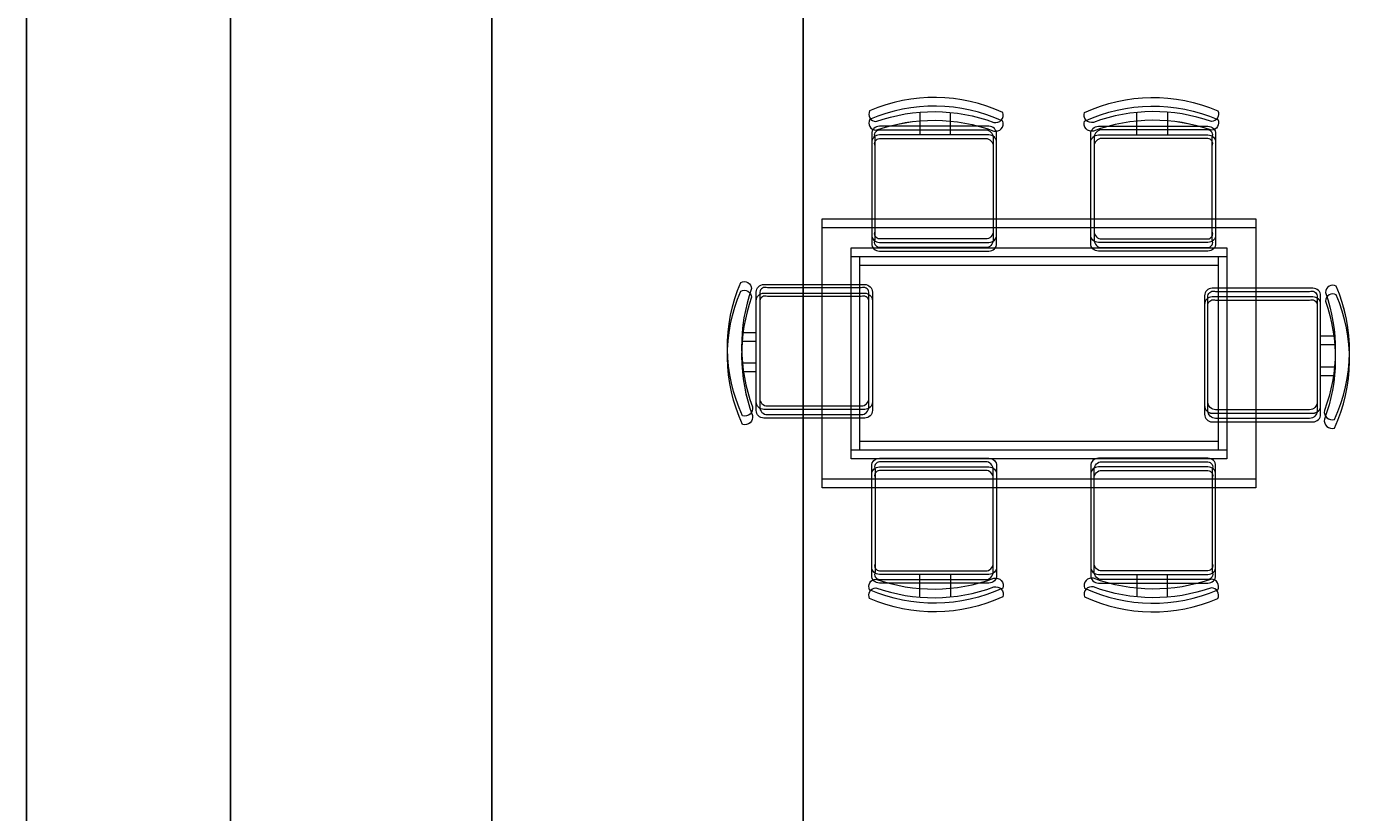
# Model space of a CAD drawing. Units: inches. Extents: x 1601 to 2297, y 1496 to 2631.
# Tile 25 of 57: x 2040 to 2141, y 1887 to 1946. Entities that reach past the tile are written whole.
import ezdxf

# ---------------------------------------------------------------- set-up
doc = ezdxf.new("R2010")
doc.units = ezdxf.units.IN
doc.layers.add('A-ANNO-DIMS', color=2, linetype='Continuous', lineweight=18)
doc.layers.add('A-FURN', color=8, linetype='Continuous', lineweight=18)
doc.styles.get("Standard").update_dxf_attribs({"font": 'arial.ttf'})
doc.dimstyles.get("Standard").update_dxf_attribs({"dimtxt": 0.18, "dimasz": 0.18, "dimexe": 0.18, "dimexo": 0.0625, "dimgap": 0.09, "dimtad": 0, "dimtih": 1, "dimtoh": 1, "dimdec": 4, "dimzin": 0, "dimdsep": 46, "dimtxsty": 'Standard', "dimcen": 0.09, "dimadec": 0, "dimazin": 0, "dimtfac": 1, "dimtdec": 4, "dimtofl": 0, "dimtmove": 0, "dimatfit": 3, "dimfxl": 1, "dimtolj": 1, "dimtzin": 0, "dimarcsym": 0})

# ---------------------------------------------------------------- blocks, each defined once
blk = doc.blocks.new('DINING-TABLE')
for points in [[(0, 20.42), (32.93, 20.42), (32.93, 0.66), (0, 0.66)], [(0, 20.42), (32.93, 20.42), (32.93, 0.66), (0, 0.66)], [(0, 20.42), (32.93, 20.42), (32.93, 0.66), (0, 0.66)], [(0, 20.42), (32.93, 20.42), (32.93, 0.66), (0, 0.66)], [(0, 19.76), (32.93, 19.76), (32.93, 0), (0, 0)], [(0, 19.76), (32.93, 19.76), (32.93, 0), (0, 0)], [(0, 19.76), (32.93, 19.76), (32.93, 0), (0, 0)], [(0, 19.76), (32.93, 19.76), (32.93, 0), (0, 0)], [(2.2, 18.22), (30.73, 18.22), (30.73, 2.85), (2.2, 2.85)], [(2.2, 18.22), (30.73, 18.22), (30.73, 2.85), (2.2, 2.85)], [(2.2, 18.22), (30.73, 18.22), (30.73, 2.85), (2.2, 2.85)], [(2.2, 18.22), (30.73, 18.22), (30.73, 2.85), (2.2, 2.85)], [(2.2, 17.56), (30.73, 17.56), (30.73, 2.2), (2.2, 2.2)], [(2.2, 17.56), (30.73, 17.56), (30.73, 2.2), (2.2, 2.2)], [(2.2, 17.56), (30.73, 17.56), (30.73, 2.2), (2.2, 2.2)], [(2.2, 17.56), (30.73, 17.56), (30.73, 2.2), (2.2, 2.2)], [(2.85, 17.56), (30.08, 17.56), (30.08, 3.51), (2.85, 3.51)], [(2.85, 17.56), (30.08, 17.56), (30.08, 3.51), (2.85, 3.51)], [(2.85, 17.56), (30.08, 17.56), (30.08, 3.51), (2.85, 3.51)], [(2.85, 17.56), (30.08, 17.56), (30.08, 3.51), (2.85, 3.51)], [(2.85, 16.9), (30.08, 16.9), (30.08, 2.85), (2.85, 2.85)], [(2.85, 16.9), (30.08, 16.9), (30.08, 2.85), (2.85, 2.85)], [(2.85, 16.9), (30.08, 16.9), (30.08, 2.85), (2.85, 2.85)], [(2.85, 16.9), (30.08, 16.9), (30.08, 2.85), (2.85, 2.85)]]:
    blk.add_lwpolyline(points, close=True)
blk = doc.blocks.new('*D39')
at = {"layer": 'A-ANNO-DIMS', "color": 0, "lineweight": -2, "transparency": 16777216}
for p, q in [((2055.55, 1981.76), (2055.55, 1513.75)), ((2099.05, 1981.76), (2099.05, 1513.75)), ((2055.73, 1513.93), (2076.97, 1513.93)), ((2098.87, 1513.93), (2077.63, 1513.93))]:
    blk.add_line(p, q, dxfattribs=at)
at = {"layer": 'A-ANNO-DIMS', "color": 0, "transparency": 16777216}
for points in [[(2055.73, 1513.96), (2055.73, 1513.9), (2055.55, 1513.93)], [(2098.87, 1513.96), (2098.87, 1513.9), (2099.05, 1513.93)]]:
    blk.add_solid(points, dxfattribs=at)
at = {"layer": 'Defpoints', "color": 0, "transparency": 16777216}
for p in [(2055.55, 1981.83), (2099.05, 1981.83), (2099.05, 1513.93)]:
    blk.add_point(p, dxfattribs=at)
at = {"layer": 'A-ANNO-DIMS', "color": 0, "transparency": 16777216, "insert": (2077.3, 1513.93), "char_height": 0.18, "attachment_point": 5}
blk.add_mtext('\\A1;43.5', dxfattribs=at)
blk = doc.blocks.new('*D41')
at = {"layer": 'A-ANNO-DIMS', "color": 0, "lineweight": -2, "transparency": 16777216}
for p, q in [((2075.4, 2070.14), (2075.4, 1513.75)), ((2040.04, 2066.51), (2040.04, 1513.75)), ((2040.22, 1513.93), (2057.32, 1513.93)), ((2075.22, 1513.93), (2058.11, 1513.93))]:
    blk.add_line(p, q, dxfattribs=at)
at = {"layer": 'A-ANNO-DIMS', "color": 0, "transparency": 16777216}
for points in [[(2040.22, 1513.96), (2040.22, 1513.9), (2040.04, 1513.93)], [(2075.22, 1513.96), (2075.22, 1513.9), (2075.4, 1513.93)]]:
    blk.add_solid(points, dxfattribs=at)
at = {"layer": 'Defpoints', "color": 0, "transparency": 16777216}
for p in [(2075.4, 2070.2), (2040.04, 2066.58), (2075.4, 1513.93)]:
    blk.add_point(p, dxfattribs=at)
at = {"layer": 'A-ANNO-DIMS', "color": 0, "transparency": 16777216, "insert": (2057.72, 1513.93), "char_height": 0.18, "attachment_point": 5}
blk.add_mtext('\\A1;35.36', dxfattribs=at)

msp = doc.modelspace()

# ---------------------------------------------------------------- linework, layer by layer
at = {"layer": 'A-FURN'}
for points in [[(2104.571, 1939.1051, -0.17580919), (2113.5401, 1939.0371, 0.57839206), (2114.2196, 1939.7843, 0.21452438), (2104.0954, 1939.9201, 0.55201397), (2104.571, 1939.1051, -0.06507904)], [(2104.571, 1939.1051, -0.17580919), (2113.5401, 1939.0371, 0.57839206), (2114.2196, 1939.7843, 0.21452438), (2104.0954, 1939.9201, 0.55201397), (2104.571, 1939.1051, -0.06507904)], [(2104.5711, 1939.1047, -0.17580919), (2113.5401, 1939.0368, 0.57839206), (2114.2196, 1939.7839, 0.21452438), (2104.0954, 1939.9198, 0.55201397), (2104.5711, 1939.1047, -0.06507904)], [(2104.5711, 1939.1047, -0.17580919), (2113.5401, 1939.0368, 0.57839206), (2114.2196, 1939.7839, 0.21452438), (2104.0954, 1939.9198, 0.55201397), (2104.5711, 1939.1047, -0.06507904)], [(2121.0909, 1939.0371, -0.57839206), (2120.4115, 1939.7843, -0.21452438), (2130.5357, 1939.9201, -0.55201397), (2130.06, 1939.1051, 0.1758092), (2121.0909, 1939.0371)], [(2121.0909, 1939.0371, -0.57839206), (2120.4115, 1939.7843, -0.21452438), (2130.5357, 1939.9201, -0.55201397), (2130.06, 1939.1051, 0.1758092), (2121.0909, 1939.0371)], [(2121.091, 1939.0368, -0.57839206), (2120.4115, 1939.7839, -0.21452438), (2130.5357, 1939.9198, -0.55201397), (2130.06, 1939.1047, 0.1758092), (2121.091, 1939.0368)], [(2121.091, 1939.0368, -0.57839206), (2120.4115, 1939.7839, -0.21452438), (2130.5357, 1939.9198, -0.55201397), (2130.06, 1939.1047, 0.1758092), (2121.091, 1939.0368)], [(2104.571, 1938.4465, -0.17580919), (2113.5401, 1938.3785, 0.57839206), (2114.2196, 1939.1257, 0.21452438), (2104.0954, 1939.2615, 0.55201397), (2104.571, 1938.4465, -0.06507904)], [(2104.571, 1938.4465, -0.17580919), (2113.5401, 1938.3785, 0.57839206), (2114.2196, 1939.1257, 0.21452438), (2104.0954, 1939.2615, 0.55201397), (2104.571, 1938.4465, -0.06507904)], [(2104.5711, 1938.4461, -0.17580919), (2113.5401, 1938.3782, 0.57839206), (2114.2196, 1939.1253, 0.21452438), (2104.0954, 1939.2612, 0.55201397), (2104.5711, 1938.4461, -0.06507904)], [(2104.5711, 1938.4461, -0.17580919), (2113.5401, 1938.3782, 0.57839206), (2114.2196, 1939.1253, 0.21452438), (2104.0954, 1939.2612, 0.55201397), (2104.5711, 1938.4461, -0.06507904)], [(2121.0909, 1938.3785, -0.57839206), (2120.4115, 1939.1257, -0.21452438), (2130.5357, 1939.2615, -0.55201397), (2130.06, 1938.4465, 0.1758092), (2121.0909, 1938.3786)], [(2121.0909, 1938.3785, -0.57839206), (2120.4115, 1939.1257, -0.21452438), (2130.5357, 1939.2615, -0.55201397), (2130.06, 1938.4465, 0.1758092), (2121.0909, 1938.3786)], [(2121.091, 1938.3782, -0.57839206), (2120.4115, 1939.1253, -0.21452438), (2130.5357, 1939.2612, -0.55201397), (2130.06, 1938.4461, 0.1758092), (2121.091, 1938.3782)], [(2121.091, 1938.3782, -0.57839206), (2120.4115, 1939.1253, -0.21452438), (2130.5357, 1939.2612, -0.55201397), (2130.06, 1938.4461, 0.1758092), (2121.091, 1938.3782)], [(2110.2349, 1938.7451), (2110.2349, 1939.7981, -0.06475861)], [(2110.2349, 1938.7451), (2110.2349, 1939.7981, -0.06475861)], [(2110.2349, 1938.7447), (2110.2349, 1939.7978, -0.06475861)], [(2110.2349, 1938.7447), (2110.2349, 1939.7978, -0.06475861)], [(2110.2349, 1938.0865), (2110.2349, 1939.1396, -0.06475861)], [(2110.2349, 1938.0865), (2110.2349, 1939.1396, -0.06475861)], [(2110.2349, 1938.0861), (2110.2349, 1939.1392, -0.06475861)], [(2110.2349, 1938.0861), (2110.2349, 1939.1392, -0.06475861)], [(2124.3962, 1938.7451), (2124.3962, 1939.7981, 0.06475861)], [(2124.3962, 1938.7451), (2124.3962, 1939.7981, 0.06475861)], [(2124.3962, 1938.7447), (2124.3962, 1939.7978, 0.06475861)], [(2124.3962, 1938.7447), (2124.3962, 1939.7978, 0.06475861)], [(2124.3962, 1938.0865), (2124.3962, 1939.1396, 0.06475861)], [(2124.3962, 1938.0865), (2124.3962, 1939.1396, 0.06475861)], [(2124.3962, 1938.0861), (2124.3962, 1939.1392, 0.06475861)], [(2124.3962, 1938.0861), (2124.3962, 1939.1392, 0.06475861)], [(2113.1596, 1938.7451), (2104.833, 1938.7451, 0.41421356), (2104.2505, 1938.1625), (2104.2505, 1930.5064, 0.41421356), (2104.833, 1929.9239), (2113.1596, 1929.9239, 0.41421356), (2113.7421, 1930.5064), (2113.7421, 1938.1625, 0.41421356), (2113.1596, 1938.7451)], [(2113.1596, 1938.7451), (2104.833, 1938.7451, 0.41421356), (2104.2505, 1938.1625), (2104.2505, 1930.5064, 0.41421356), (2104.833, 1929.9239), (2113.1596, 1929.9239, 0.41421356), (2113.7421, 1930.5064), (2113.7421, 1938.1625, 0.41421356), (2113.1596, 1938.7451)], [(2113.1596, 1938.7447), (2104.833, 1938.7447, 0.41421356), (2104.2505, 1938.1622), (2104.2505, 1930.5061, 0.41421356), (2104.833, 1929.9235), (2113.1596, 1929.9235, 0.41421356), (2113.7422, 1930.5061), (2113.7422, 1938.1622, 0.41421356), (2113.1596, 1938.7447)], [(2113.1596, 1938.7447), (2104.833, 1938.7447, 0.41421356), (2104.2505, 1938.1622), (2104.2505, 1930.5061, 0.41421356), (2104.833, 1929.9235), (2113.1596, 1929.9235, 0.41421356), (2113.7422, 1930.5061), (2113.7422, 1938.1622, 0.41421356), (2113.1596, 1938.7447)], [(2113.1596, 1938.0865), (2104.833, 1938.0865, 0.41421356), (2104.2505, 1937.504), (2104.2505, 1929.8478, 0.41421356), (2104.833, 1929.2653), (2113.1596, 1929.2653, 0.41421356), (2113.7421, 1929.8478), (2113.7421, 1937.504, 0.41421356), (2113.1596, 1938.0865)], [(2113.1596, 1938.0865), (2104.833, 1938.0865, 0.41421356), (2104.2505, 1937.504), (2104.2505, 1929.8478, 0.41421356), (2104.833, 1929.2653), (2113.1596, 1929.2653, 0.41421356), (2113.7421, 1929.8478), (2113.7421, 1937.504, 0.41421356), (2113.1596, 1938.0865)], [(2113.1596, 1938.0861), (2104.833, 1938.0861, 0.41421356), (2104.2505, 1937.5036), (2104.2505, 1929.8475, 0.41421356), (2104.833, 1929.2649), (2113.1596, 1929.2649, 0.41421356), (2113.7422, 1929.8475), (2113.7422, 1937.5036, 0.41421356), (2113.1596, 1938.0861)], [(2113.1596, 1938.0861), (2104.833, 1938.0861, 0.41421356), (2104.2505, 1937.5036), (2104.2505, 1929.8475, 0.41421356), (2104.833, 1929.2649), (2113.1596, 1929.2649, 0.41421356), (2113.7422, 1929.8475), (2113.7422, 1937.5036, 0.41421356), (2113.1596, 1938.0861)], [(2129.798, 1938.7451, -0.41421356), (2130.3806, 1938.1625), (2130.3806, 1930.5064, -0.41421356), (2129.798, 1929.9239), (2121.4715, 1929.9239, -0.41421356), (2120.8889, 1930.5064), (2120.8889, 1938.1625, -0.41421356), (2121.4715, 1938.7451), (2129.798, 1938.7451)], [(2129.798, 1938.7451, -0.41421356), (2130.3806, 1938.1625), (2130.3806, 1930.5064, -0.41421356), (2129.798, 1929.9239), (2121.4715, 1929.9239, -0.41421356), (2120.8889, 1930.5064), (2120.8889, 1938.1625, -0.41421356), (2121.4715, 1938.7451), (2129.798, 1938.7451)], [(2129.7981, 1938.7447, -0.41421356), (2130.3806, 1938.1622), (2130.3806, 1930.5061, -0.41421356), (2129.7981, 1929.9235), (2121.4715, 1929.9235, -0.41421356), (2120.8889, 1930.5061), (2120.8889, 1938.1622, -0.41421356), (2121.4715, 1938.7447), (2129.7981, 1938.7447)], [(2129.7981, 1938.7447, -0.41421356), (2130.3806, 1938.1622), (2130.3806, 1930.5061, -0.41421356), (2129.7981, 1929.9235), (2121.4715, 1929.9235, -0.41421356), (2120.8889, 1930.5061), (2120.8889, 1938.1622, -0.41421356), (2121.4715, 1938.7447), (2129.7981, 1938.7447)], [(2129.798, 1938.0865, -0.41421356), (2130.3806, 1937.504), (2130.3806, 1929.8478, -0.41421356), (2129.798, 1929.2653), (2121.4715, 1929.2653, -0.41421356), (2120.8889, 1929.8478), (2120.8889, 1937.504, -0.41421356), (2121.4715, 1938.0865), (2129.798, 1938.0865)], [(2129.798, 1938.0865, -0.41421356), (2130.3806, 1937.504), (2130.3806, 1929.8478, -0.41421356), (2129.798, 1929.2653), (2121.4715, 1929.2653, -0.41421356), (2120.8889, 1929.8478), (2120.8889, 1937.504, -0.41421356), (2121.4715, 1938.0865), (2129.798, 1938.0865)], [(2129.7981, 1938.0861, -0.41421356), (2130.3806, 1937.5036), (2130.3806, 1929.8475, -0.41421356), (2129.7981, 1929.2649), (2121.4715, 1929.2649, -0.41421356), (2120.8889, 1929.8475), (2120.8889, 1937.5036, -0.41421356), (2121.4715, 1938.0861), (2129.7981, 1938.0861)], [(2129.7981, 1938.0861, -0.41421356), (2130.3806, 1937.5036), (2130.3806, 1929.8475, -0.41421356), (2129.7981, 1929.2649), (2121.4715, 1929.2649, -0.41421356), (2120.8889, 1929.8475), (2120.8889, 1937.5036, -0.41421356), (2121.4715, 1938.0861), (2129.7981, 1938.0861)], [(2095.1877, 1917.4461, -0.57839206), (2094.4405, 1916.7666, -0.21452438), (2094.3047, 1926.8908, -0.55201397), (2095.1197, 1926.4152, 0.17580937), (2095.1877, 1917.4461)], [(2095.1877, 1917.4461, -0.57839206), (2094.4405, 1916.7666, -0.21452438), (2094.3047, 1926.8908, -0.55201397), (2095.1197, 1926.4152, 0.17580937), (2095.1877, 1917.4461)], [(2095.1877, 1917.4457, -0.57839206), (2094.4405, 1916.7663, -0.21452438), (2094.3047, 1926.8905, -0.55201397), (2095.1198, 1926.4148, 0.17580937), (2095.1877, 1917.4457)], [(2095.1877, 1917.4457, -0.57839206), (2094.4405, 1916.7663, -0.21452438), (2094.3047, 1926.8905, -0.55201397), (2095.1198, 1926.4148, 0.17580937), (2095.1877, 1917.4457)], [(2095.1877, 1916.7875, -0.57839206), (2094.4405, 1916.108, -0.21452438), (2094.3047, 1926.2322, -0.55201397), (2095.1197, 1925.7566, 0.17580937), (2095.1877, 1916.7875)], [(2095.1877, 1916.7875, -0.57839206), (2094.4405, 1916.108, -0.21452438), (2094.3047, 1926.2322, -0.55201397), (2095.1197, 1925.7566, 0.17580937), (2095.1877, 1916.7875)], [(2095.1877, 1916.7872, -0.57839206), (2094.4405, 1916.1077, -0.21452438), (2094.3047, 1926.2319, -0.55201397), (2095.1198, 1925.7562, 0.17580937), (2095.1877, 1916.7871)], [(2095.1877, 1916.7872, -0.57839206), (2094.4405, 1916.1077, -0.21452438), (2094.3047, 1926.2319, -0.55201397), (2095.1198, 1925.7562, 0.17580937), (2095.1877, 1916.7871)], [(2095.4797, 1926.1532, -0.41421356), (2096.0623, 1926.7357), (2103.7184, 1926.7357, -0.41421356), (2104.3009, 1926.1532), (2104.3009, 1917.8266, -0.41421356), (2103.7184, 1917.2441), (2096.0623, 1917.2441, -0.41421356), (2095.4797, 1917.8266), (2095.4797, 1926.1532)], [(2095.4797, 1926.1532, -0.41421356), (2096.0623, 1926.7357), (2103.7184, 1926.7357, -0.41421356), (2104.3009, 1926.1532), (2104.3009, 1917.8266, -0.41421356), (2103.7184, 1917.2441), (2096.0623, 1917.2441, -0.41421356), (2095.4797, 1917.8266), (2095.4797, 1926.1532)], [(2095.4797, 1926.1529, -0.41421356), (2096.0623, 1926.7354), (2103.7184, 1926.7354, -0.41421356), (2104.301, 1926.1529), (2104.301, 1917.8263, -0.41421356), (2103.7184, 1917.2437), (2096.0623, 1917.2437, -0.41421356), (2095.4797, 1917.8263), (2095.4797, 1926.1529)], [(2095.4797, 1926.1529, -0.41421356), (2096.0623, 1926.7354), (2103.7184, 1926.7354, -0.41421356), (2104.301, 1926.1529), (2104.301, 1917.8263, -0.41421356), (2103.7184, 1917.2437), (2096.0623, 1917.2437, -0.41421356), (2095.4797, 1917.8263), (2095.4797, 1926.1529)], [(2095.4797, 1925.4946, -0.41421356), (2096.0623, 1926.0771), (2103.7184, 1926.0771, -0.41421356), (2104.3009, 1925.4946), (2104.3009, 1917.168, -0.41421356), (2103.7184, 1916.5855), (2096.0623, 1916.5855, -0.41421356), (2095.4797, 1917.168), (2095.4797, 1925.4946)], [(2095.4797, 1925.4946, -0.41421356), (2096.0623, 1926.0771), (2103.7184, 1926.0771, -0.41421356), (2104.3009, 1925.4946), (2104.3009, 1917.168, -0.41421356), (2103.7184, 1916.5855), (2096.0623, 1916.5855, -0.41421356), (2095.4797, 1917.168), (2095.4797, 1925.4946)], [(2095.4797, 1925.4943, -0.41421356), (2096.0623, 1926.0768), (2103.7184, 1926.0768, -0.41421356), (2104.301, 1925.4943), (2104.301, 1917.1677, -0.41421356), (2103.7184, 1916.5851), (2096.0623, 1916.5851, -0.41421356), (2095.4797, 1917.1677), (2095.4797, 1925.4943)], [(2095.4797, 1925.4943, -0.41421356), (2096.0623, 1926.0768), (2103.7184, 1926.0768, -0.41421356), (2104.301, 1925.4943), (2104.301, 1917.1677, -0.41421356), (2103.7184, 1916.5851), (2096.0623, 1916.5851, -0.41421356), (2095.4797, 1917.1677), (2095.4797, 1925.4943)], [(2138.3578, 1925.868, 0.41421356), (2137.7752, 1926.4506), (2130.1191, 1926.4506, 0.41421356), (2129.5366, 1925.868), (2129.5366, 1917.5414, 0.41421356), (2130.1191, 1916.9589), (2137.7752, 1916.9589, 0.41421356), (2138.3578, 1917.5414), (2138.3578, 1925.868)], [(2138.3578, 1925.868, 0.41421356), (2137.7752, 1926.4506), (2130.1191, 1926.4506, 0.41421356), (2129.5366, 1925.868), (2129.5366, 1917.5414, 0.41421356), (2130.1191, 1916.9589), (2137.7752, 1916.9589, 0.41421356), (2138.3578, 1917.5414), (2138.3578, 1925.868)], [(2138.3578, 1925.8677, 0.41421356), (2137.7753, 1926.4502), (2130.1191, 1926.4502, 0.41421356), (2129.5366, 1925.8677), (2129.5366, 1917.5411, 0.41421356), (2130.1191, 1916.9586), (2137.7753, 1916.9586, 0.41421356), (2138.3578, 1917.5411), (2138.3578, 1925.8677)], [(2138.3578, 1925.8677, 0.41421356), (2137.7753, 1926.4502), (2130.1191, 1926.4502, 0.41421356), (2129.5366, 1925.8677), (2129.5366, 1917.5411, 0.41421356), (2130.1191, 1916.9586), (2137.7753, 1916.9586, 0.41421356), (2138.3578, 1917.5411), (2138.3578, 1925.8677)], [(2138.7178, 1926.13, -0.17580919), (2138.6498, 1917.1609, 0.57839206), (2139.397, 1916.4814, 0.21452438), (2139.5328, 1926.6056, 0.55201397), (2138.7178, 1926.13, -0.06507904)], [(2138.7178, 1926.13, -0.17580919), (2138.6498, 1917.1609, 0.57839206), (2139.397, 1916.4814, 0.21452438), (2139.5328, 1926.6056, 0.55201397), (2138.7178, 1926.13, -0.06507904)], [(2138.7178, 1926.1297, -0.17580919), (2138.6499, 1917.1606, 0.57839206), (2139.397, 1916.4811, 0.21452438), (2139.5328, 1926.6053, 0.55201397), (2138.7178, 1926.1297, -0.06507904)], [(2138.7178, 1926.1297, -0.17580919), (2138.6499, 1917.1606, 0.57839206), (2139.397, 1916.4811, 0.21452438), (2139.5328, 1926.6053, 0.55201397), (2138.7178, 1926.1297, -0.06507904)], [(2138.7178, 1925.4714, -0.17580919), (2138.6498, 1916.5023, 0.57839206), (2139.397, 1915.8229, 0.21452438), (2139.5328, 1925.947, 0.55201397), (2138.7178, 1925.4714, -0.06507904)], [(2138.7178, 1925.4714, -0.17580919), (2138.6498, 1916.5023, 0.57839206), (2139.397, 1915.8229, 0.21452438), (2139.5328, 1925.947, 0.55201397), (2138.7178, 1925.4714, -0.06507904)], [(2138.7178, 1925.4711, -0.17580919), (2138.6499, 1916.502, 0.57839206), (2139.397, 1915.8225, 0.21452438), (2139.5328, 1925.9467, 0.55201397), (2138.7178, 1925.4711, -0.06507904)], [(2138.7178, 1925.4711, -0.17580919), (2138.6499, 1916.502, 0.57839206), (2139.397, 1915.8225, 0.21452438), (2139.5328, 1925.9467, 0.55201397), (2138.7178, 1925.4711, -0.06507904)], [(2138.3578, 1925.2094, 0.41421356), (2137.7752, 1925.792), (2130.1191, 1925.792, 0.41421356), (2129.5366, 1925.2094), (2129.5366, 1916.8828, 0.41421356), (2130.1191, 1916.3003), (2137.7752, 1916.3003, 0.41421356), (2138.3578, 1916.8828), (2138.3578, 1925.2094)], [(2138.3578, 1925.2094, 0.41421356), (2137.7752, 1925.792), (2130.1191, 1925.792, 0.41421356), (2129.5366, 1925.2094), (2129.5366, 1916.8828, 0.41421356), (2130.1191, 1916.3003), (2137.7752, 1916.3003, 0.41421356), (2138.3578, 1916.8828), (2138.3578, 1925.2094)], [(2138.3578, 1925.2091, 0.41421356), (2137.7753, 1925.7916), (2130.1191, 1925.7916, 0.41421356), (2129.5366, 1925.2091), (2129.5366, 1916.8825, 0.41421356), (2130.1191, 1916.3), (2137.7753, 1916.3, 0.41421356), (2138.3578, 1916.8825), (2138.3578, 1925.2091)], [(2138.3578, 1925.2091, 0.41421356), (2137.7753, 1925.7916), (2130.1191, 1925.7916, 0.41421356), (2129.5366, 1925.2091), (2129.5366, 1916.8825, 0.41421356), (2130.1191, 1916.3), (2137.7753, 1916.3, 0.41421356), (2138.3578, 1916.8825), (2138.3578, 1925.2091)], [(2095.4797, 1920.7513), (2094.4267, 1920.7513, 0.06475861)], [(2095.4797, 1920.7513), (2094.4267, 1920.7513, 0.06475861)], [(2095.4797, 1920.751), (2094.4267, 1920.751, 0.06475861)], [(2095.4797, 1920.751), (2094.4267, 1920.751, 0.06475861)], [(2095.4797, 1920.0927), (2094.4267, 1920.0927, 0.06475861)], [(2095.4797, 1920.0927), (2094.4267, 1920.0927, 0.06475861)], [(2095.4797, 1920.0924), (2094.4267, 1920.0924, 0.06475861)], [(2095.4797, 1920.0924), (2094.4267, 1920.0924, 0.06475861)], [(2138.3578, 1920.4662), (2139.4108, 1920.4662, -0.06475861)], [(2138.3578, 1920.4662), (2139.4108, 1920.4662, -0.06475861)], [(2138.3578, 1920.4658), (2139.4109, 1920.4658, -0.06475861)], [(2138.3578, 1920.4658), (2139.4109, 1920.4658, -0.06475861)], [(2138.3578, 1919.8076), (2139.4108, 1919.8076, -0.06475861)], [(2138.3578, 1919.8076), (2139.4108, 1919.8076, -0.06475861)], [(2138.3578, 1919.8072), (2139.4109, 1919.8072, -0.06475861)], [(2138.3578, 1919.8072), (2139.4109, 1919.8072, -0.06475861)], [(2113.1596, 1904.7117), (2104.833, 1904.7117, -0.41421356), (2104.2505, 1905.2942), (2104.2505, 1912.9503, -0.41421356), (2104.833, 1913.5329), (2113.1596, 1913.5329, -0.41421356), (2113.7421, 1912.9503), (2113.7421, 1905.2942, -0.41421356), (2113.1596, 1904.7117)], [(2113.1596, 1904.7117), (2104.833, 1904.7117, -0.41421356), (2104.2505, 1905.2942), (2104.2505, 1912.9503, -0.41421356), (2104.833, 1913.5329), (2113.1596, 1913.5329, -0.41421356), (2113.7421, 1912.9503), (2113.7421, 1905.2942, -0.41421356), (2113.1596, 1904.7117)], [(2113.1596, 1904.7113), (2104.833, 1904.7113, -0.41421356), (2104.2505, 1905.2939), (2104.2505, 1912.95, -0.41421356), (2104.833, 1913.5325), (2113.1596, 1913.5325, -0.41421356), (2113.7422, 1912.95), (2113.7422, 1905.2939, -0.41421356), (2113.1596, 1904.7113)], [(2113.1596, 1904.7113), (2104.833, 1904.7113, -0.41421356), (2104.2505, 1905.2939), (2104.2505, 1912.95, -0.41421356), (2104.833, 1913.5325), (2113.1596, 1913.5325, -0.41421356), (2113.7422, 1912.95), (2113.7422, 1905.2939, -0.41421356), (2113.1596, 1904.7113)], [(2113.1596, 1904.0531), (2104.833, 1904.0531, -0.41421356), (2104.2505, 1904.6356), (2104.2505, 1912.2917, -0.41421356), (2104.833, 1912.8743), (2113.1596, 1912.8743, -0.41421356), (2113.7421, 1912.2917), (2113.7421, 1904.6356, -0.41421356), (2113.1596, 1904.0531)], [(2113.1596, 1904.0531), (2104.833, 1904.0531, -0.41421356), (2104.2505, 1904.6356), (2104.2505, 1912.2917, -0.41421356), (2104.833, 1912.8743), (2113.1596, 1912.8743, -0.41421356), (2113.7421, 1912.2917), (2113.7421, 1904.6356, -0.41421356), (2113.1596, 1904.0531)], [(2113.1596, 1904.0527), (2104.833, 1904.0527, -0.41421356), (2104.2505, 1904.6353), (2104.2505, 1912.2914, -0.41421356), (2104.833, 1912.8739), (2113.1596, 1912.8739, -0.41421356), (2113.7422, 1912.2914), (2113.7422, 1904.6353, -0.41421356), (2113.1596, 1904.0527)], [(2113.1596, 1904.0527), (2104.833, 1904.0527, -0.41421356), (2104.2505, 1904.6353), (2104.2505, 1912.2914, -0.41421356), (2104.833, 1912.8739), (2113.1596, 1912.8739, -0.41421356), (2113.7422, 1912.2914), (2113.7422, 1904.6353, -0.41421356), (2113.1596, 1904.0527)], [(2129.798, 1904.7117, 0.41421356), (2130.3806, 1905.2942), (2130.3806, 1912.9503, 0.41421356), (2129.798, 1913.5329), (2121.4715, 1913.5329, 0.41421356), (2120.8889, 1912.9503), (2120.8889, 1905.2942, 0.41421356), (2121.4715, 1904.7117), (2129.798, 1904.7117)], [(2129.798, 1904.7117, 0.41421356), (2130.3806, 1905.2942), (2130.3806, 1912.9503, 0.41421356), (2129.798, 1913.5329), (2121.4715, 1913.5329, 0.41421356), (2120.8889, 1912.9503), (2120.8889, 1905.2942, 0.41421356), (2121.4715, 1904.7117), (2129.798, 1904.7117)], [(2129.7981, 1904.7113, 0.41421356), (2130.3806, 1905.2939), (2130.3806, 1912.95, 0.41421356), (2129.7981, 1913.5325), (2121.4715, 1913.5325, 0.41421356), (2120.8889, 1912.95), (2120.8889, 1905.2939, 0.41421356), (2121.4715, 1904.7113), (2129.7981, 1904.7113)], [(2129.7981, 1904.7113, 0.41421356), (2130.3806, 1905.2939), (2130.3806, 1912.95, 0.41421356), (2129.7981, 1913.5325), (2121.4715, 1913.5325, 0.41421356), (2120.8889, 1912.95), (2120.8889, 1905.2939, 0.41421356), (2121.4715, 1904.7113), (2129.7981, 1904.7113)], [(2129.798, 1904.0531, 0.41421356), (2130.3806, 1904.6356), (2130.3806, 1912.2917, 0.41421356), (2129.798, 1912.8743), (2121.4715, 1912.8743, 0.41421356), (2120.8889, 1912.2917), (2120.8889, 1904.6356, 0.41421356), (2121.4715, 1904.0531), (2129.798, 1904.0531)], [(2129.798, 1904.0531, 0.41421356), (2130.3806, 1904.6356), (2130.3806, 1912.2917, 0.41421356), (2129.798, 1912.8743), (2121.4715, 1912.8743, 0.41421356), (2120.8889, 1912.2917), (2120.8889, 1904.6356, 0.41421356), (2121.4715, 1904.0531), (2129.798, 1904.0531)], [(2129.7981, 1904.0527, 0.41421356), (2130.3806, 1904.6353), (2130.3806, 1912.2914, 0.41421356), (2129.7981, 1912.8739), (2121.4715, 1912.8739, 0.41421356), (2120.8889, 1912.2914), (2120.8889, 1904.6353, 0.41421356), (2121.4715, 1904.0527), (2129.7981, 1904.0527)], [(2129.7981, 1904.0527, 0.41421356), (2130.3806, 1904.6353), (2130.3806, 1912.2914, 0.41421356), (2129.7981, 1912.8739), (2121.4715, 1912.8739, 0.41421356), (2120.8889, 1912.2914), (2120.8889, 1904.6353, 0.41421356), (2121.4715, 1904.0527), (2129.7981, 1904.0527)], [(2113.5401, 1904.4196, -0.57839206), (2114.2196, 1903.6725, -0.21452438), (2104.0954, 1903.5366, -0.55201397), (2104.571, 1904.3517, 0.17580929), (2113.5401, 1904.4196)], [(2113.5401, 1904.4196, -0.57839206), (2114.2196, 1903.6725, -0.21452438), (2104.0954, 1903.5366, -0.55201397), (2104.571, 1904.3517, 0.17580929), (2113.5401, 1904.4196)], [(2113.5401, 1904.4193, -0.57839206), (2114.2196, 1903.6721, -0.21452438), (2104.0954, 1903.5363, -0.55201397), (2104.5711, 1904.3513, 0.17580929), (2113.5401, 1904.4193)], [(2113.5401, 1904.4193, -0.57839206), (2114.2196, 1903.6721, -0.21452438), (2104.0954, 1903.5363, -0.55201397), (2104.5711, 1904.3513, 0.17580929), (2113.5401, 1904.4193)], [(2113.5401, 1903.761, -0.57839206), (2114.2196, 1903.0139, -0.21452438), (2104.0954, 1902.878, -0.55201397), (2104.571, 1903.6931, 0.17580929), (2113.5401, 1903.761)], [(2113.5401, 1903.761, -0.57839206), (2114.2196, 1903.0139, -0.21452438), (2104.0954, 1902.878, -0.55201397), (2104.571, 1903.6931, 0.17580929), (2113.5401, 1903.761)], [(2113.5401, 1903.7607, -0.57839206), (2114.2196, 1903.0135, -0.21452438), (2104.0954, 1902.8777, -0.55201397), (2104.5711, 1903.6927, 0.17580929), (2113.5401, 1903.7607)], [(2113.5401, 1903.7607, -0.57839206), (2114.2196, 1903.0135, -0.21452438), (2104.0954, 1902.8777, -0.55201397), (2104.5711, 1903.6927, 0.17580929), (2113.5401, 1903.7607)], [(2110.2349, 1904.7117), (2110.2349, 1903.6586, 0.06475861)], [(2110.2349, 1904.7117), (2110.2349, 1903.6586, 0.06475861)], [(2110.2349, 1904.7113), (2110.2349, 1903.6583, 0.06475861)], [(2110.2349, 1904.7113), (2110.2349, 1903.6583, 0.06475861)], [(2110.2349, 1904.0531), (2110.2349, 1903, 0.06475861)], [(2110.2349, 1904.0531), (2110.2349, 1903, 0.06475861)], [(2110.2349, 1904.0527), (2110.2349, 1902.9997, 0.06475861)], [(2110.2349, 1904.0527), (2110.2349, 1902.9997, 0.06475861)], [(2130.06, 1904.3517, -0.17580928), (2121.0909, 1904.4196, 0.57839206), (2120.4115, 1903.6725, 0.21452438), (2130.5357, 1903.5366, 0.55201397), (2130.06, 1904.3517, -0.06507904)], [(2130.06, 1904.3517, -0.17580928), (2121.0909, 1904.4196, 0.57839206), (2120.4115, 1903.6725, 0.21452438), (2130.5357, 1903.5366, 0.55201397), (2130.06, 1904.3517, -0.06507904)], [(2130.06, 1904.3513, -0.17580928), (2121.091, 1904.4193, 0.57839206), (2120.4115, 1903.6721, 0.21452438), (2130.5357, 1903.5363, 0.55201397), (2130.06, 1904.3513, -0.06507904)], [(2130.06, 1904.3513, -0.17580928), (2121.091, 1904.4193, 0.57839206), (2120.4115, 1903.6721, 0.21452438), (2130.5357, 1903.5363, 0.55201397), (2130.06, 1904.3513, -0.06507904)], [(2130.06, 1903.6931, -0.17580928), (2121.0909, 1903.761, 0.57839206), (2120.4115, 1903.0139, 0.21452438), (2130.5357, 1902.878, 0.55201397), (2130.06, 1903.6931, -0.06507904)], [(2130.06, 1903.6931, -0.17580928), (2121.0909, 1903.761, 0.57839206), (2120.4115, 1903.0139, 0.21452438), (2130.5357, 1902.878, 0.55201397), (2130.06, 1903.6931, -0.06507904)], [(2130.06, 1903.6927, -0.17580928), (2121.091, 1903.7607, 0.57839206), (2120.4115, 1903.0135, 0.21452438), (2130.5357, 1902.8777, 0.55201397), (2130.06, 1903.6927, -0.06507904)], [(2130.06, 1903.6927, -0.17580928), (2121.091, 1903.7607, 0.57839206), (2120.4115, 1903.0135, 0.21452438), (2130.5357, 1902.8777, 0.55201397), (2130.06, 1903.6927, -0.06507904)], [(2124.3962, 1904.7117), (2124.3962, 1903.6586, -0.06475861)], [(2124.3962, 1904.7117), (2124.3962, 1903.6586, -0.06475861)], [(2124.3962, 1904.7113), (2124.3962, 1903.6583, -0.06475861)], [(2124.3962, 1904.7113), (2124.3962, 1903.6583, -0.06475861)], [(2124.3962, 1904.0531), (2124.3962, 1903, -0.06475861)], [(2124.3962, 1904.0531), (2124.3962, 1903, -0.06475861)], [(2124.3962, 1904.0527), (2124.3962, 1902.9997, -0.06475861)], [(2124.3962, 1904.0527), (2124.3962, 1902.9997, -0.06475861)]]:
    msp.add_lwpolyline(points, format="xyb", dxfattribs=at)
for points in [[(2107.9042, 1939.8173), (2107.9042, 1938.7451)], [(2107.9042, 1939.8173), (2107.9042, 1938.7451)], [(2107.9042, 1939.8169), (2107.9042, 1938.7447)], [(2107.9042, 1939.8169), (2107.9042, 1938.7447)], [(2107.9042, 1939.1587), (2107.9042, 1938.0865)], [(2107.9042, 1939.1587), (2107.9042, 1938.0865)], [(2107.9042, 1939.1583), (2107.9042, 1938.0861)], [(2107.9042, 1939.1583), (2107.9042, 1938.0861)], [(2126.7269, 1939.8173), (2126.7269, 1938.7451)], [(2126.7269, 1939.8173), (2126.7269, 1938.7451)], [(2126.7269, 1939.8169), (2126.7269, 1938.7447)], [(2126.7269, 1939.8169), (2126.7269, 1938.7447)], [(2126.7269, 1939.1587), (2126.7269, 1938.0865)], [(2126.7269, 1939.1587), (2126.7269, 1938.0865)], [(2126.7269, 1939.1583), (2126.7269, 1938.0861)], [(2126.7269, 1939.1583), (2126.7269, 1938.0861)], [(2094.4075, 1923.0821), (2095.4797, 1923.0821)], [(2094.4075, 1923.0821), (2095.4797, 1923.0821)], [(2094.4075, 1923.0817), (2095.4797, 1923.0817)], [(2094.4075, 1923.0817), (2095.4797, 1923.0817)], [(2094.4075, 1922.4235), (2095.4797, 1922.4235)], [(2094.4075, 1922.4235), (2095.4797, 1922.4235)], [(2094.4075, 1922.4231), (2095.4797, 1922.4231)], [(2094.4075, 1922.4231), (2095.4797, 1922.4231)], [(2139.43, 1922.7969), (2138.3578, 1922.7969)], [(2139.43, 1922.7969), (2138.3578, 1922.7969)], [(2139.43, 1922.7965), (2138.3578, 1922.7965)], [(2139.43, 1922.7965), (2138.3578, 1922.7965)], [(2139.43, 1922.1383), (2138.3578, 1922.1383)], [(2139.43, 1922.1383), (2138.3578, 1922.1383)], [(2139.43, 1922.138), (2138.3578, 1922.138)], [(2139.43, 1922.138), (2138.3578, 1922.138)], [(2107.9042, 1903.6395), (2107.9042, 1904.7117)], [(2107.9042, 1903.6395), (2107.9042, 1904.7117)], [(2107.9042, 1903.6391), (2107.9042, 1904.7113)], [(2107.9042, 1903.6391), (2107.9042, 1904.7113)], [(2107.9042, 1902.9809), (2107.9042, 1904.0531)], [(2107.9042, 1902.9809), (2107.9042, 1904.0531)], [(2107.9042, 1902.9805), (2107.9042, 1904.0527)], [(2107.9042, 1902.9805), (2107.9042, 1904.0527)], [(2126.7269, 1903.6395), (2126.7269, 1904.7117)], [(2126.7269, 1903.6395), (2126.7269, 1904.7117)], [(2126.7269, 1903.6391), (2126.7269, 1904.7113)], [(2126.7269, 1903.6391), (2126.7269, 1904.7113)], [(2126.7269, 1902.9809), (2126.7269, 1904.0531)], [(2126.7269, 1902.9809), (2126.7269, 1904.0531)], [(2126.7269, 1902.9805), (2126.7269, 1904.0527)], [(2126.7269, 1902.9805), (2126.7269, 1904.0527)]]:
    msp.add_lwpolyline(points, dxfattribs=at)
for points in [[(2104.8365, 1938.4826), (2112.8972, 1938.4826, -0.41421356), (2113.4797, 1937.9001), (2113.4797, 1930.7688, -0.41421356), (2112.8972, 1930.1863), (2104.8365, 1930.1863, -0.51206948), (2104.5129, 1930.7688), (2104.5129, 1937.9001, -0.51206948)], [(2104.8365, 1938.4826), (2112.8972, 1938.4826, -0.41421356), (2113.4797, 1937.9001), (2113.4797, 1930.7688, -0.41421356), (2112.8972, 1930.1863), (2104.8365, 1930.1863, -0.51206948), (2104.5129, 1930.7688), (2104.5129, 1937.9001, -0.51206948)], [(2104.8366, 1938.4823), (2112.8972, 1938.4823, -0.41421356), (2113.4797, 1937.8998), (2113.4797, 1930.7685, -0.41421356), (2112.8972, 1930.186), (2104.8366, 1930.186, -0.51206948), (2104.5129, 1930.7685), (2104.5129, 1937.8998, -0.51206948)], [(2104.8366, 1938.4823), (2112.8972, 1938.4823, -0.41421356), (2113.4797, 1937.8998), (2113.4797, 1930.7685, -0.41421356), (2112.8972, 1930.186), (2104.8366, 1930.186, -0.51206948), (2104.5129, 1930.7685), (2104.5129, 1937.8998, -0.51206948)], [(2129.7945, 1938.4826), (2121.7339, 1938.4826, 0.41421356), (2121.1514, 1937.9001), (2121.1514, 1930.7688, 0.41421356), (2121.7339, 1930.1863), (2129.7945, 1930.1863, 0.51206948), (2130.1181, 1930.7688), (2130.1181, 1937.9001, 0.51206948)], [(2129.7945, 1938.4826), (2121.7339, 1938.4826, 0.41421356), (2121.1514, 1937.9001), (2121.1514, 1930.7688, 0.41421356), (2121.7339, 1930.1863), (2129.7945, 1930.1863, 0.51206948), (2130.1181, 1930.7688), (2130.1181, 1937.9001, 0.51206948)], [(2129.7945, 1938.4823), (2121.7339, 1938.4823, 0.41421356), (2121.1514, 1937.8998), (2121.1514, 1930.7685, 0.41421356), (2121.7339, 1930.186), (2129.7945, 1930.186, 0.51206948), (2130.1182, 1930.7685), (2130.1182, 1937.8998, 0.51206948)], [(2129.7945, 1938.4823), (2121.7339, 1938.4823, 0.41421356), (2121.1514, 1937.8998), (2121.1514, 1930.7685, 0.41421356), (2121.7339, 1930.186), (2129.7945, 1930.186, 0.51206948), (2130.1182, 1930.7685), (2130.1182, 1937.8998, 0.51206948)], [(2104.8365, 1937.8241), (2112.8972, 1937.8241, -0.41421356), (2113.4797, 1937.2415), (2113.4797, 1930.1103, -0.41421356), (2112.8972, 1929.5277), (2104.8365, 1929.5277, -0.51206948), (2104.5129, 1930.1103), (2104.5129, 1937.2415, -0.51206948)], [(2104.8365, 1937.8241), (2112.8972, 1937.8241, -0.41421356), (2113.4797, 1937.2415), (2113.4797, 1930.1103, -0.41421356), (2112.8972, 1929.5277), (2104.8365, 1929.5277, -0.51206948), (2104.5129, 1930.1103), (2104.5129, 1937.2415, -0.51206948)], [(2104.8366, 1937.8237), (2112.8972, 1937.8237, -0.41421356), (2113.4797, 1937.2412), (2113.4797, 1930.1099, -0.41421356), (2112.8972, 1929.5274), (2104.8366, 1929.5274, -0.51206948), (2104.5129, 1930.1099), (2104.5129, 1937.2412, -0.51206948)], [(2104.8366, 1937.8237), (2112.8972, 1937.8237, -0.41421356), (2113.4797, 1937.2412), (2113.4797, 1930.1099, -0.41421356), (2112.8972, 1929.5274), (2104.8366, 1929.5274, -0.51206948), (2104.5129, 1930.1099), (2104.5129, 1937.2412, -0.51206948)], [(2129.7945, 1937.8241), (2121.7339, 1937.8241, 0.41421356), (2121.1514, 1937.2415), (2121.1514, 1930.1103, 0.41421356), (2121.7339, 1929.5277), (2129.7945, 1929.5277, 0.51206948), (2130.1181, 1930.1103), (2130.1181, 1937.2415, 0.51206948)], [(2129.7945, 1937.8241), (2121.7339, 1937.8241, 0.41421356), (2121.1514, 1937.2415), (2121.1514, 1930.1103, 0.41421356), (2121.7339, 1929.5277), (2129.7945, 1929.5277, 0.51206948), (2130.1181, 1930.1103), (2130.1181, 1937.2415, 0.51206948)], [(2129.7945, 1937.8237), (2121.7339, 1937.8237, 0.41421356), (2121.1514, 1937.2412), (2121.1514, 1930.1099, 0.41421356), (2121.7339, 1929.5274), (2129.7945, 1929.5274, 0.51206948), (2130.1182, 1930.1099), (2130.1182, 1937.2412, 0.51206948)], [(2129.7945, 1937.8237), (2121.7339, 1937.8237, 0.41421356), (2121.1514, 1937.2412), (2121.1514, 1930.1099, 0.41421356), (2121.7339, 1929.5274), (2129.7945, 1929.5274, 0.51206948), (2130.1182, 1930.1099), (2130.1182, 1937.2412, 0.51206948)], [(2095.7422, 1926.1497), (2095.7422, 1918.089, 0.41421356), (2096.3247, 1917.5065), (2103.456, 1917.5065, 0.41421356), (2104.0385, 1918.089), (2104.0385, 1926.1497, 0.51206948), (2103.456, 1926.4733), (2096.3247, 1926.4733, 0.51206948)], [(2095.7422, 1926.1497), (2095.7422, 1918.089, 0.41421356), (2096.3247, 1917.5065), (2103.456, 1917.5065, 0.41421356), (2104.0385, 1918.089), (2104.0385, 1926.1497, 0.51206948), (2103.456, 1926.4733), (2096.3247, 1926.4733, 0.51206948)], [(2095.7422, 1926.1493), (2095.7422, 1918.0887, 0.41421356), (2096.3247, 1917.5062), (2103.456, 1917.5062, 0.41421356), (2104.0385, 1918.0887), (2104.0385, 1926.1493, 0.51206948), (2103.456, 1926.473), (2096.3247, 1926.473, 0.51206948)], [(2095.7422, 1926.1493), (2095.7422, 1918.0887, 0.41421356), (2096.3247, 1917.5062), (2103.456, 1917.5062, 0.41421356), (2104.0385, 1918.0887), (2104.0385, 1926.1493, 0.51206948), (2103.456, 1926.473), (2096.3247, 1926.473, 0.51206948)], [(2138.0953, 1925.8645), (2138.0953, 1917.8039, -0.41421356), (2137.5128, 1917.2213), (2130.3815, 1917.2213, -0.41421356), (2129.799, 1917.8039), (2129.799, 1925.8645, -0.51206948), (2130.3815, 1926.1881), (2137.5128, 1926.1881, -0.51206948)], [(2138.0953, 1925.8645), (2138.0953, 1917.8039, -0.41421356), (2137.5128, 1917.2213), (2130.3815, 1917.2213, -0.41421356), (2129.799, 1917.8039), (2129.799, 1925.8645, -0.51206948), (2130.3815, 1926.1881), (2137.5128, 1926.1881, -0.51206948)], [(2138.0954, 1925.8642), (2138.0954, 1917.8035, -0.41421356), (2137.5128, 1917.221), (2130.3816, 1917.221, -0.41421356), (2129.799, 1917.8035), (2129.799, 1925.8642, -0.51206948), (2130.3816, 1926.1878), (2137.5128, 1926.1878, -0.51206948)], [(2138.0954, 1925.8642), (2138.0954, 1917.8035, -0.41421356), (2137.5128, 1917.221), (2130.3816, 1917.221, -0.41421356), (2129.799, 1917.8035), (2129.799, 1925.8642, -0.51206948), (2130.3816, 1926.1878), (2137.5128, 1926.1878, -0.51206948)], [(2095.7422, 1925.4911), (2095.7422, 1917.4305, 0.41421356), (2096.3247, 1916.8479), (2103.456, 1916.8479, 0.41421356), (2104.0385, 1917.4305), (2104.0385, 1925.4911, 0.51206948), (2103.456, 1925.8147), (2096.3247, 1925.8147, 0.51206948)], [(2095.7422, 1925.4911), (2095.7422, 1917.4305, 0.41421356), (2096.3247, 1916.8479), (2103.456, 1916.8479, 0.41421356), (2104.0385, 1917.4305), (2104.0385, 1925.4911, 0.51206948), (2103.456, 1925.8147), (2096.3247, 1925.8147, 0.51206948)], [(2095.7422, 1925.4907), (2095.7422, 1917.4301, 0.41421356), (2096.3247, 1916.8476), (2103.456, 1916.8476, 0.41421356), (2104.0385, 1917.4301), (2104.0385, 1925.4907, 0.51206948), (2103.456, 1925.8144), (2096.3247, 1925.8144, 0.51206948)], [(2095.7422, 1925.4907), (2095.7422, 1917.4301, 0.41421356), (2096.3247, 1916.8476), (2103.456, 1916.8476, 0.41421356), (2104.0385, 1917.4301), (2104.0385, 1925.4907, 0.51206948), (2103.456, 1925.8144), (2096.3247, 1925.8144, 0.51206948)], [(2138.0953, 1925.2059), (2138.0953, 1917.1453, -0.41421356), (2137.5128, 1916.5627), (2130.3815, 1916.5627, -0.41421356), (2129.799, 1917.1453), (2129.799, 1925.2059, -0.51206948), (2130.3815, 1925.5295), (2137.5128, 1925.5295, -0.51206948)], [(2138.0953, 1925.2059), (2138.0953, 1917.1453, -0.41421356), (2137.5128, 1916.5627), (2130.3815, 1916.5627, -0.41421356), (2129.799, 1917.1453), (2129.799, 1925.2059, -0.51206948), (2130.3815, 1925.5295), (2137.5128, 1925.5295, -0.51206948)], [(2138.0954, 1925.2056), (2138.0954, 1917.1449, -0.41421356), (2137.5128, 1916.5624), (2130.3816, 1916.5624, -0.41421356), (2129.799, 1917.1449), (2129.799, 1925.2056, -0.51206948), (2130.3816, 1925.5292), (2137.5128, 1925.5292, -0.51206948)], [(2138.0954, 1925.2056), (2138.0954, 1917.1449, -0.41421356), (2137.5128, 1916.5624), (2130.3816, 1916.5624, -0.41421356), (2129.799, 1917.1449), (2129.799, 1925.2056, -0.51206948), (2130.3816, 1925.5292), (2137.5128, 1925.5292, -0.51206948)], [(2104.8365, 1904.9741), (2112.8972, 1904.9741, 0.41421356), (2113.4797, 1905.5566), (2113.4797, 1912.6879, 0.41421356), (2112.8972, 1913.2704), (2104.8365, 1913.2704, 0.51206948), (2104.5129, 1912.6879), (2104.5129, 1905.5566, 0.51206948)], [(2104.8365, 1904.9741), (2112.8972, 1904.9741, 0.41421356), (2113.4797, 1905.5566), (2113.4797, 1912.6879, 0.41421356), (2112.8972, 1913.2704), (2104.8365, 1913.2704, 0.51206948), (2104.5129, 1912.6879), (2104.5129, 1905.5566, 0.51206948)], [(2104.8366, 1904.9738), (2112.8972, 1904.9738, 0.41421356), (2113.4797, 1905.5563), (2113.4797, 1912.6876, 0.41421356), (2112.8972, 1913.2701), (2104.8366, 1913.2701, 0.51206948), (2104.5129, 1912.6876), (2104.5129, 1905.5563, 0.51206948)], [(2104.8366, 1904.9738), (2112.8972, 1904.9738, 0.41421356), (2113.4797, 1905.5563), (2113.4797, 1912.6876, 0.41421356), (2112.8972, 1913.2701), (2104.8366, 1913.2701, 0.51206948), (2104.5129, 1912.6876), (2104.5129, 1905.5563, 0.51206948)], [(2129.7945, 1904.9741), (2121.7339, 1904.9741, -0.41421356), (2121.1514, 1905.5566), (2121.1514, 1912.6879, -0.41421356), (2121.7339, 1913.2704), (2129.7945, 1913.2704, -0.51206948), (2130.1181, 1912.6879), (2130.1181, 1905.5566, -0.51206948)], [(2129.7945, 1904.9741), (2121.7339, 1904.9741, -0.41421356), (2121.1514, 1905.5566), (2121.1514, 1912.6879, -0.41421356), (2121.7339, 1913.2704), (2129.7945, 1913.2704, -0.51206948), (2130.1181, 1912.6879), (2130.1181, 1905.5566, -0.51206948)], [(2129.7945, 1904.9738), (2121.7339, 1904.9738, -0.41421356), (2121.1514, 1905.5563), (2121.1514, 1912.6876, -0.41421356), (2121.7339, 1913.2701), (2129.7945, 1913.2701, -0.51206948), (2130.1182, 1912.6876), (2130.1182, 1905.5563, -0.51206948)], [(2129.7945, 1904.9738), (2121.7339, 1904.9738, -0.41421356), (2121.1514, 1905.5563), (2121.1514, 1912.6876, -0.41421356), (2121.7339, 1913.2701), (2129.7945, 1913.2701, -0.51206948), (2130.1182, 1912.6876), (2130.1182, 1905.5563, -0.51206948)], [(2104.8365, 1904.3155), (2112.8972, 1904.3155, 0.41421356), (2113.4797, 1904.898), (2113.4797, 1912.0293, 0.41421356), (2112.8972, 1912.6118), (2104.8365, 1912.6118, 0.51206948), (2104.5129, 1912.0293), (2104.5129, 1904.898, 0.51206948)], [(2104.8365, 1904.3155), (2112.8972, 1904.3155, 0.41421356), (2113.4797, 1904.898), (2113.4797, 1912.0293, 0.41421356), (2112.8972, 1912.6118), (2104.8365, 1912.6118, 0.51206948), (2104.5129, 1912.0293), (2104.5129, 1904.898, 0.51206948)], [(2104.8366, 1904.3152), (2112.8972, 1904.3152, 0.41421356), (2113.4797, 1904.8977), (2113.4797, 1912.029, 0.41421356), (2112.8972, 1912.6115), (2104.8366, 1912.6115, 0.51206948), (2104.5129, 1912.029), (2104.5129, 1904.8977, 0.51206948)], [(2104.8366, 1904.3152), (2112.8972, 1904.3152, 0.41421356), (2113.4797, 1904.8977), (2113.4797, 1912.029, 0.41421356), (2112.8972, 1912.6115), (2104.8366, 1912.6115, 0.51206948), (2104.5129, 1912.029), (2104.5129, 1904.8977, 0.51206948)], [(2129.7945, 1904.3155), (2121.7339, 1904.3155, -0.41421356), (2121.1514, 1904.898), (2121.1514, 1912.0293, -0.41421356), (2121.7339, 1912.6118), (2129.7945, 1912.6118, -0.51206948), (2130.1181, 1912.0293), (2130.1181, 1904.898, -0.51206948)], [(2129.7945, 1904.3155), (2121.7339, 1904.3155, -0.41421356), (2121.1514, 1904.898), (2121.1514, 1912.0293, -0.41421356), (2121.7339, 1912.6118), (2129.7945, 1912.6118, -0.51206948), (2130.1181, 1912.0293), (2130.1181, 1904.898, -0.51206948)], [(2129.7945, 1904.3152), (2121.7339, 1904.3152, -0.41421356), (2121.1514, 1904.8977), (2121.1514, 1912.029, -0.41421356), (2121.7339, 1912.6115), (2129.7945, 1912.6115, -0.51206948), (2130.1182, 1912.029), (2130.1182, 1904.8977, -0.51206948)], [(2129.7945, 1904.3152), (2121.7339, 1904.3152, -0.41421356), (2121.1514, 1904.8977), (2121.1514, 1912.029, -0.41421356), (2121.7339, 1912.6115), (2129.7945, 1912.6115, -0.51206948), (2130.1182, 1912.029), (2130.1182, 1904.8977, -0.51206948)]]:
    msp.add_lwpolyline(points, format="xyb", close=True, dxfattribs=at)

# ---------------------------------------------------------------- block references
msp.add_blockref('DINING-TABLE', (2100.4975, 1911.2966), dxfattribs=at)

# ---------------------------------------------------------------- dimensions: what is measured, and where the dimension line sits
at = {"layer": 'A-ANNO-DIMS'}
for base, p1, p2, override, picture, middle in [((2075.3977, 1513.9279), (2040.0373, 2066.5754), (2075.3977, 2070.1988), {"dimdec": 2, "dimlfac": 1, "dimrnd": 0, "dimzin": 0, "dimdsep": 46, "dimlunit": 2}, '*D41', (2057.7175, 1513.9279)), ((2099.05, 1513.9279), (2055.5513, 1981.8254), (2099.05, 1981.8254), {"dimdec": 1, "dimlfac": 1, "dimrnd": 0, "dimzin": 0, "dimdsep": 46, "dimlunit": 2}, '*D39', (2077.3006, 1513.9279))]:
    dim = msp.add_linear_dim(base=base, p1=p1, p2=p2, dimstyle='Standard', override=override, dxfattribs=at)
    dim.commit()
    dim.dimension.update_dxf_attribs({"geometry": picture, "text_midpoint": middle})

doc.saveas('drawing.dxf')
